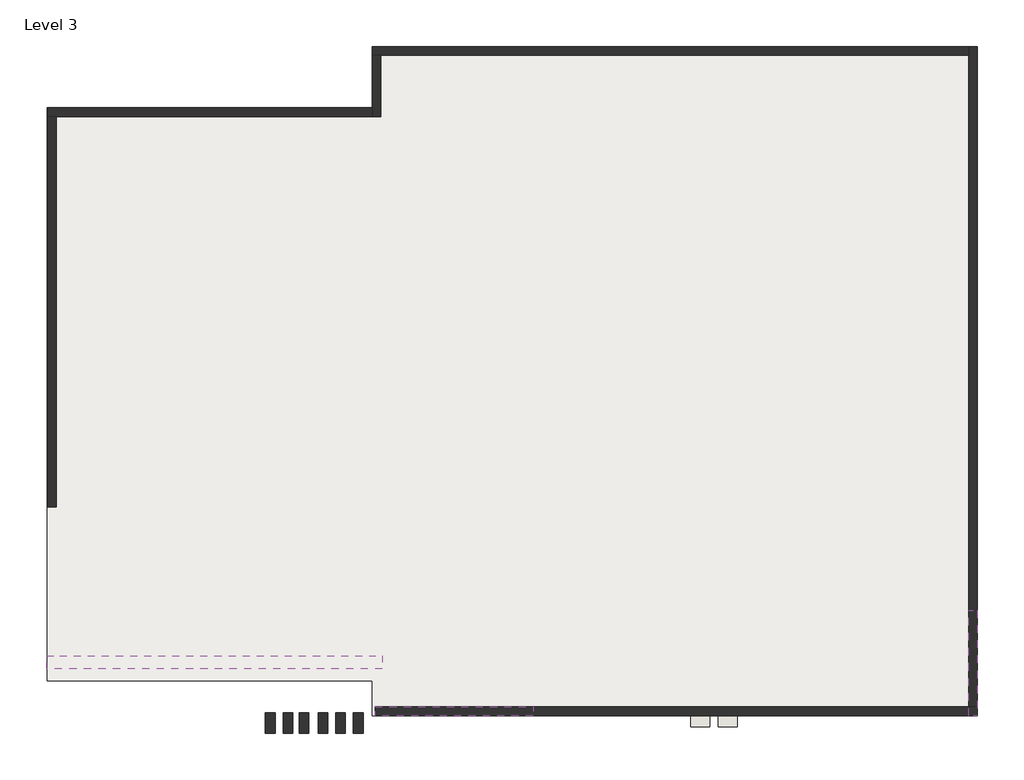
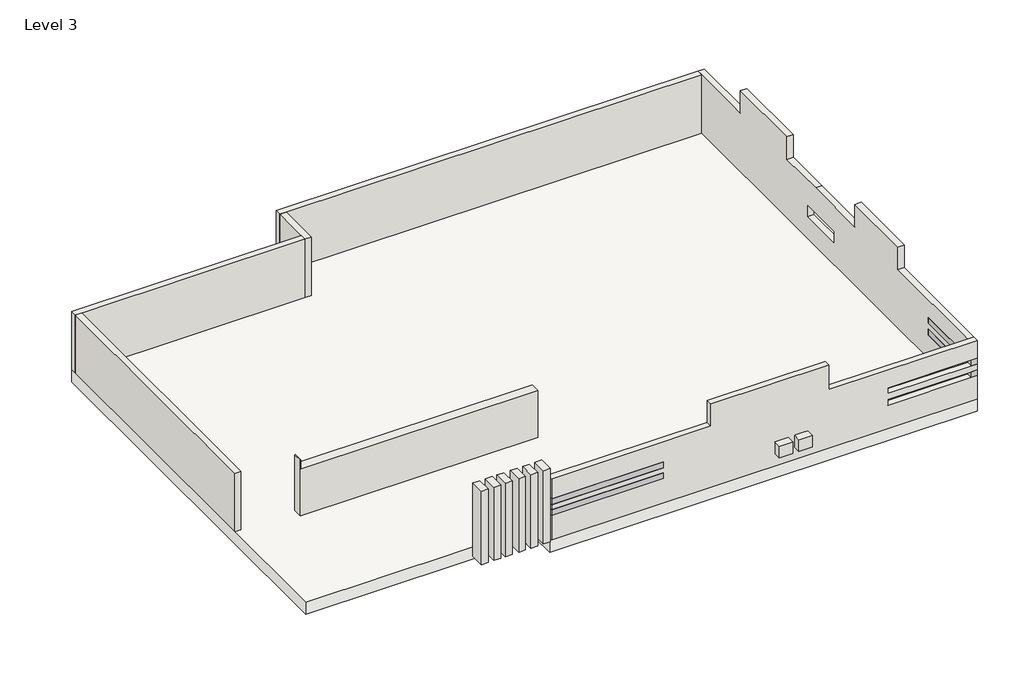
# One storey: 9 walls, 4 proxies, 1 roof.
"""IFC4 building model written with IfcOpenShell, lengths in millimetres."""

from ifc_helpers import new_model, si_unit, frame, origin, place, context, project, spatial, polyline, outline, extrude, faceted_brep, transform, mapped, element, save
from components import walls_3_walls_3_68a7d47a, walls_9_walls_9_54edce94

model = new_model("IFC4")

# Units and contexts
model_context = context("Model", 3, world=origin())
ifc_project = project(units=[si_unit("LENGTHUNIT", "METRE", prefix="MILLI")], contexts=[model_context])

# Site, building, storey
site = spatial("IfcSite", under=ifc_project)
building = spatial("IfcBuilding", under=site)
storey = spatial("IfcBuildingStorey", under=building, Name="Level 3", Elevation=7315.2)

# Proxies
placement = place(None, origin())
element("IfcBuildingElementProxy", 1, Name="Reveal", ObjectType="Reveal", at=placement, inside=storey, context=model_context, shape_type="SweptSolid", body=[
    extrude(outline(polyline([(2348.6271302, -3701.0259649), (2196.2271302, -3701.0259649), (2196.2271302, -1872.2259649), (2348.6271302, -1872.2259649), (2348.6271302, -3701.0259649)])), frame((0.0, 0.0, 8534.4), z_axis=(0.0, 0.0, 1.0), x_axis=(1.0, 0.0, 0.0)), (0.0, 0.0, 1.0), 152.4),
])
element("IfcBuildingElementProxy", 2, Name="Reveal", ObjectType="Reveal", at=placement, inside=storey, context=model_context, shape_type="SweptSolid", body=[
    extrude(outline(polyline([(-8116.1728698, -3701.0259649), (-8116.1728698, -3548.6259649), (-5372.9728698, -3548.6259649), (-5372.9728698, -3701.0259649), (-8116.1728698, -3701.0259649)])), frame((0.0, 0.0, 8536.4737715), z_axis=(0.0, 0.0, 1.0), x_axis=(1.0, 0.0, 0.0)), (0.0, 0.0, 1.0), 152.4),
])
element("IfcBuildingElementProxy", 3, Name="Reveal", ObjectType="Reveal", at=placement, inside=storey, context=model_context, shape_type="SweptSolid", body=[
    extrude(outline(polyline([(-8116.1728698, -3701.0259649), (-8116.1728698, -3548.6259649), (-5372.9728698, -3548.6259649), (-5372.9728698, -3701.0259649), (-8116.1728698, -3701.0259649)])), frame((0.0, 0.0, 8255.0001399), z_axis=(0.0, 0.0, 1.0), x_axis=(1.0, 0.0, 0.0)), (0.0, 0.0, 1.0), 152.4),
])
element("IfcBuildingElementProxy", 4, Name="Reveal", ObjectType="Reveal", at=placement, inside=storey, context=model_context, shape_type="SweptSolid", body=[
    extrude(outline(polyline([(2348.6271302, -3701.0259649), (2196.2271302, -3701.0259649), (2196.2271302, -1872.2259649), (2348.6271302, -1872.2259649), (2348.6271302, -3701.0259649)])), frame((0.0, 0.0, 8229.6), z_axis=(0.0, 0.0, 1.0), x_axis=(1.0, 0.0, 0.0)), (0.0, 0.0, 1.0), 152.4),
])

# Roof
element("IfcRoof", 5, ObjectType="Generic - 12\"", at=placement, inside=storey, context=model_context, shape_type="SweptSolid", body=[
    extrude(outline(polyline([(-13813.3305193, 6865.3740351), (-8166.9728698, 6865.3740351), (-8166.9728698, 7932.1740351), (2348.6271302, 7932.1740351), (2348.6271302, -3701.0259649), (-8166.9728698, -3701.0259649), (-8166.9728698, -3091.4259649), (-13813.3305193, -3091.4259649), (-13813.3305193, 6865.3740351)])), frame((0.0, 0.0, 7315.2), z_axis=(0.0, 0.0, 1.0), x_axis=(1.0, 0.0, 0.0)), (0.0, 0.0, 1.0), 304.8),
])

# Walls
element("IfcWall", 6, ObjectType="Generic - 6\"", at=placement, inside=storey, context=model_context, shape_type="Brep", body=[
    faceted_brep([(2348.6271302, -3701.0259649, 9144.0), (-1308.9728698, -3701.0259649, 9144.0), (-1308.9728698, -3701.0259649, 9785.7694166), (-4204.5728698, -3701.0259649, 9785.7694166), (-4204.5728698, -3701.0259649, 9212.8470483), (-8116.1728698, -3701.0259649, 9212.8470483), (-8116.1728698, -3701.0259649, 8688.8737715), (-5372.9728698, -3701.0259649, 8688.8737715), (-5372.9728698, -3701.0259649, 8536.4737715), (-8116.1728698, -3701.0259649, 8536.4737715), (-8116.1728698, -3701.0259649, 8407.4001399), (-5372.9728698, -3701.0259649, 8407.4001399), (-5372.9728698, -3701.0259649, 8255.0001399), (-8116.1728698, -3701.0259649, 8255.0001399), (-8116.1728698, -3701.0259649, 7617.5521516), (2348.6271302, -3701.0259649, 7617.5521516), (2348.6271302, -3701.0259649, 8229.6), (2196.2271302, -3701.0259649, 8229.6), (138.8271302, -3701.0259649, 8229.6), (138.8271302, -3701.0259649, 8380.7760758), (2196.2271302, -3701.0259649, 8380.7760758), (2196.2271302, -3701.0259649, 8382.0), (2348.6271302, -3701.0259649, 8382.0), (2348.6271302, -3701.0259649, 8534.4), (2196.2271302, -3701.0259649, 8534.4), (138.8271302, -3701.0259649, 8534.4), (138.8271302, -3701.0259649, 8686.8), (2196.2271302, -3701.0259649, 8686.8), (2348.6271302, -3701.0259649, 8686.8), (-1308.9728698, -3548.6259649, 9144.0), (2196.2271302, -3548.6259649, 9144.0), (2348.6271302, -3548.6259649, 9144.0), (2348.6271302, -3548.6259649, 8686.8), (2196.2271302, -3548.6259649, 8686.8), (138.8271302, -3548.6259649, 8686.8), (138.8271302, -3548.6259649, 8534.4), (2196.2271302, -3548.6259649, 8534.4), (2348.6271302, -3548.6259649, 8534.4), (2348.6271302, -3548.6259649, 8382.0), (2196.2271302, -3548.6259649, 8382.0), (2196.2271302, -3548.6259649, 8380.7760758), (138.8271302, -3548.6259649, 8380.7760758), (138.8271302, -3548.6259649, 8229.6), (2196.2271302, -3548.6259649, 8229.6), (2348.6271302, -3548.6259649, 8229.6), (2348.6271302, -3548.6259649, 7620.0), (2348.6271302, -3548.6259649, 7617.5521516), (-8116.1728698, -3548.6259649, 7617.5521516), (-8116.1728698, -3548.6259649, 8255.0001399), (-5372.9728698, -3548.6259649, 8255.0001399), (-5372.9728698, -3548.6259649, 8407.4001399), (-8116.1728698, -3548.6259649, 8407.4001399), (-8116.1728698, -3548.6259649, 8536.4737715), (-5372.9728698, -3548.6259649, 8536.4737715), (-5372.9728698, -3548.6259649, 8688.8737715), (-8116.1728698, -3548.6259649, 8688.8737715), (-8116.1728698, -3548.6259649, 9212.8470483), (-4204.5728698, -3548.6259649, 9212.8470483), (-4204.5728698, -3548.6259649, 9785.7694166), (-1308.9728698, -3548.6259649, 9785.7694166)], [[[0, 1, 2, 3, 4, 5, 6, 7, 8, 9, 10, 11, 12, 13, 14, 15, 16, 17, 18, 19, 20, 21, 22, 23, 24, 25, 26, 27, 28]], [[29, 30, 31, 32, 33, 34, 35, 36, 37, 38, 39, 40, 41, 42, 43, 44, 45, 46, 47, 48, 49, 50, 51, 52, 53, 54, 55, 56, 57, 58, 59]], [[1, 0, 31, 30, 29]], [[2, 1, 29, 59]], [[3, 2, 59, 58]], [[4, 3, 58, 57]], [[5, 4, 57, 56]], [[15, 14, 47, 46]], [[53, 8, 7, 54]], [[54, 7, 6, 55]], [[8, 53, 52, 9]], [[49, 12, 11, 50]], [[50, 11, 10, 51]], [[12, 49, 48, 13]], [[5, 56, 55, 6]], [[47, 14, 13, 48]], [[51, 10, 9, 52]], [[21, 39, 38, 22]], [[39, 21, 20, 40]], [[42, 18, 17, 16, 44, 43]], [[19, 18, 42, 41]], [[19, 41, 40, 20]], [[35, 25, 24, 23, 37, 36]], [[26, 25, 35, 34]], [[26, 34, 33, 32, 28, 27]], [[16, 15, 46, 45, 44]], [[37, 23, 22, 38]], [[0, 28, 32, 31]]]),
])
element("IfcWall", 7, ObjectType="Generic - 6\"", at=placement, inside=storey, context=model_context, shape_type="Brep", body=[
    faceted_brep([(2348.6271302, -3548.6259649, 7620.0), (2348.6271302, 7932.1740351, 7620.0), (2348.6271302, 7932.1740351, 9144.0), (2348.6271302, 6128.7740351, 9144.0), (2348.6271302, 6128.7740351, 9731.3133194), (2348.6271302, 4147.5740351, 9731.3133194), (2348.6271302, 4147.5740351, 9144.0), (2348.6271302, 2928.3740351, 9144.0), (2348.6271302, 1251.9740351, 9144.0), (2348.6271302, 1251.9740351, 9731.3133194), (2348.6271302, -576.8259649, 9731.3133194), (2348.6271302, -576.8259649, 9144.0), (2348.6271302, -3548.6259649, 9144.0), (2348.6271302, -3548.6259649, 8686.8), (2348.6271302, -1872.2259649, 8686.8), (2348.6271302, -1872.2259649, 8534.4), (2348.6271302, -3548.6259649, 8534.4), (2348.6271302, -3548.6259649, 8382.0), (2348.6271302, -1872.2259649, 8382.0), (2348.6271302, -1872.2259649, 8229.6), (2348.6271302, -3548.6259649, 8229.6), (2348.6271302, 3260.506606, 8479.0034325), (2348.6271302, 3260.506606, 8199.6034325), (2348.6271302, 2142.906606, 8199.6034325), (2348.6271302, 2142.906606, 8479.0034325), (2196.2271302, 7932.1740351, 7620.0), (2196.2271302, 7779.7740351, 7620.0), (2196.2271302, -3548.6259649, 7620.0), (2196.2271302, -3548.6259649, 8229.6), (2196.2271302, -1872.2259649, 8229.6), (2196.2271302, -1872.2259649, 8382.0), (2196.2271302, -3548.6259649, 8382.0), (2196.2271302, -3548.6259649, 8534.4), (2196.2271302, -1872.2259649, 8534.4), (2196.2271302, -1872.2259649, 8686.8), (2196.2271302, -3548.6259649, 8686.8), (2196.2271302, -3548.6259649, 9144.0), (2196.2271302, -576.8259649, 9144.0), (2196.2271302, -576.8259649, 9731.3133194), (2196.2271302, 1251.9740351, 9731.3133194), (2196.2271302, 1251.9740351, 9144.0), (2196.2271302, 2928.3740351, 9144.0), (2196.2271302, 4147.5740351, 9144.0), (2196.2271302, 4147.5740351, 9731.3133194), (2196.2271302, 6128.7740351, 9731.3133194), (2196.2271302, 6128.7740351, 9144.0), (2196.2271302, 7779.7740351, 9144.0), (2196.2271302, 7932.1740351, 9144.0), (2196.2271302, 3260.506606, 8199.6034325), (2196.2271302, 3260.506606, 8479.0034325), (2196.2271302, 2142.906606, 8479.0034325), (2196.2271302, 2142.906606, 8199.6034325)], [[[0, 1, 2, 3, 4, 5, 6, 7, 8, 9, 10, 11, 12, 13, 14, 15, 16, 17, 18, 19, 20], [21, 22, 23, 24]], [[25, 26, 27, 28, 29, 30, 31, 32, 33, 34, 35, 36, 37, 38, 39, 40, 41, 42, 43, 44, 45, 46, 47], [48, 49, 50, 51]], [[2, 1, 25, 47]], [[1, 0, 27, 26, 25]], [[12, 11, 37, 36]], [[33, 15, 14, 34]], [[34, 14, 13, 35]], [[15, 33, 32, 16]], [[3, 2, 47, 46, 45]], [[4, 3, 45, 44]], [[5, 4, 44, 43]], [[6, 5, 43, 42]], [[7, 6, 42, 41]], [[8, 7, 41, 40]], [[9, 8, 40, 39]], [[10, 9, 39, 38]], [[11, 10, 38, 37]], [[29, 19, 18, 30]], [[30, 18, 17, 31]], [[19, 29, 28, 20]], [[27, 0, 20, 28]], [[12, 36, 35, 13]], [[16, 32, 31, 17]], [[22, 21, 49, 48]], [[23, 22, 48, 51]], [[24, 23, 51, 50]], [[21, 24, 50, 49]]]),
])
element("IfcWall", 8, ObjectType="Generic - 6\"", at=placement, inside=storey, context=model_context, shape_type="Brep", body=[
    faceted_brep([(2196.2271302, 7932.1740351, 7620.0), (-8166.9728698, 7932.1740351, 7620.0), (-8166.9728698, 7932.1740351, 9144.0), (2196.2271302, 7932.1740351, 9144.0), (2196.2271302, 7779.7740351, 7620.0), (2196.2271302, 7779.7740351, 9144.0), (-8014.5728698, 7779.7740351, 9144.0), (-8166.9728698, 7779.7740351, 9144.0), (-8166.9728698, 7779.7740351, 7620.0), (-8014.5728698, 7779.7740351, 7620.0)], [[[0, 1, 2, 3]], [[4, 5, 6, 7, 8, 9]], [[0, 3, 5, 4]], [[2, 1, 8, 7]], [[1, 0, 4, 9, 8]], [[3, 2, 7, 6, 5]]]),
])
element("IfcWall", 9, ObjectType="Generic - 6\"", at=placement, inside=storey, context=model_context, shape_type="Brep", body=[
    faceted_brep([(-8166.9728698, 7779.7740351, 7620.0), (-8166.9728698, 6865.3740351, 7620.0), (-8166.9728698, 6712.9740351, 7620.0), (-8166.9728698, 6712.9740351, 9144.0), (-8166.9728698, 6865.3740351, 9144.0), (-8166.9728698, 7779.7740351, 9144.0), (-8014.5728698, 7779.7740351, 7620.0), (-8014.5728698, 7779.7740351, 9144.0), (-8014.5728698, 6712.9740351, 9144.0), (-8014.5728698, 6712.9740351, 7620.0)], [[[0, 1, 2, 3, 4, 5]], [[6, 7, 8, 9]], [[2, 1, 0, 6, 9]], [[5, 4, 3, 8, 7]], [[0, 5, 7, 6]], [[3, 2, 9, 8]]]),
])
element("IfcWall", 10, ObjectType="Generic - 6\"", at=placement, inside=storey, context=model_context, shape_type="Brep", body=[
    faceted_brep([(-8166.9728698, 6865.3740351, 7620.0), (-13806.9805193, 6865.3740351, 7620.0), (-13806.9805193, 6865.3740351, 9144.0), (-8166.9728698, 6865.3740351, 9144.0), (-8166.9728698, 6712.9740351, 7620.0), (-8166.9728698, 6712.9740351, 9144.0), (-13654.5805193, 6712.9740351, 9144.0), (-13806.9805193, 6712.9740351, 9144.0), (-13806.9805193, 6712.9740351, 7620.0), (-13654.5805193, 6712.9740351, 7620.0)], [[[0, 1, 2, 3]], [[4, 5, 6, 7, 8, 9]], [[1, 0, 4, 9, 8]], [[3, 2, 7, 6, 5]], [[0, 3, 5, 4]], [[2, 1, 8, 7]]]),
])
element("IfcWall", 11, ObjectType="Generic - 6\"", at=placement, inside=storey, context=model_context, shape_type="SweptSolid", body=[
    extrude(outline(polyline([(-13806.9805193, -68.8259649), (-13806.9805193, 6712.9740351), (-13654.5805193, 6712.9740351), (-13654.5805193, -68.8259649), (-13806.9805193, -68.8259649)])), frame((0.0, 0.0, 7620.0), z_axis=(0.0, 0.0, 1.0), x_axis=(1.0, 0.0, 0.0)), (0.0, 0.0, 1.0), 1524.0),
])
element("IfcWall", 12, ObjectType="Generic - 8\" - Filled", at=placement, inside=storey, context=model_context, shape_type="Brep", body=[
    faceted_brep([(-13824.8228698, -2888.2259649, 9753.6), (-7989.1728698, -2888.2259649, 9753.6), (-7989.1728698, -2888.2259649, 10972.8), (-13810.1555193, -2888.2259649, 10972.8), (-13810.1555193, -2888.2259649, 11202.4428486), (-13824.8228698, -2888.2259649, 11202.4428486), (-13824.8228698, -2659.6259649, 9753.6), (-13824.8228698, -2659.6259649, 11194.4859918), (-13824.8228698, -2659.6259649, 11202.4428486), (-13810.1555193, -2659.6259649, 11202.4428486), (-13810.1555193, -2659.6259649, 11194.4859918), (-13810.1555193, -2659.6259649, 10972.8), (-13596.2228698, -2659.6259649, 10972.8), (-8217.7728698, -2659.6259649, 10972.8), (-7989.1728698, -2659.6259649, 10972.8), (-7989.1728698, -2659.6259649, 9753.6), (-13596.2228698, -2659.6259649, 9753.6)], [[[0, 1, 2, 3, 4, 5]], [[6, 7, 8, 9, 10, 11, 12, 13, 14, 15, 16]], [[1, 0, 6, 16, 15]], [[0, 5, 8, 7, 6]], [[2, 1, 15, 14]], [[5, 4, 9, 8]], [[9, 4, 3, 11, 10]], [[3, 2, 14, 13, 12, 11]]]),
])
walls_3_walls_3_shape = walls_3_walls_3_68a7d47a(model_context)
element("IfcWall", 13, ObjectType="Walls 3 : Walls 3", at=placement, inside=storey, context=model_context, shape_type="MappedRepresentation", body=[
    mapped(walls_3_walls_3_shape, transform((0.0, 0.0, 0.0), x_axis=(1.0, 0.0, 0.0), y_axis=(0.0, 1.0, 0.0), z_axis=(0.0, 0.0, 1.0))),
])
walls_9_walls_9_shape = walls_9_walls_9_54edce94(model_context)
element("IfcWall", 14, ObjectType="Walls 9 : Walls 9", at=placement, inside=storey, context=model_context, shape_type="MappedRepresentation", body=[
    mapped(walls_9_walls_9_shape, transform((0.0, 0.0, 0.0), x_axis=(1.0, 0.0, 0.0), y_axis=(0.0, 1.0, 0.0), z_axis=(0.0, 0.0, 1.0))),
])

save(model, "model.ifc")

# Revit data of these elements
# Type "Generic - 12\""
#   Assembly Code = "B1020"
#   Layers, outside or top first: 1' - 0" no material (function 1)
# Type "Generic - 6\""
#   Assembly Code = "B2010"
#   Layers, outside or top first: 0' - 6" no material (function 1)
# Type "Generic - 8\" - Filled"
#   Assembly Code = "B2010"
#   Layers, outside or top first: 0' - 9" no material (function 1)
# Element 5 (IfcRoof, "Generic - 12\"")
#   built-in parameter 1001705 = 25 (stored number, unit not read)
#   built-in parameter 1001710 = 33615
#   Phase Created = New Construction
#   Materials on its faces: "Default Roof"
# Element 6 (IfcWall, "Generic - 6\"")
#   built-in parameter 1001111 = 1' - 0"
#   Top Offset = 0' - 0"
#   Base Offset = 1' - 0"
#   Unconnected Height = 5' - 2.71051"
#   wall height = 5' - 2.71051"
#   Phase Created = New Construction
#   Base Constraint = Level 3
#   Materials on its faces: "Default Wall"
# Elements 7, 8, 9, 10, 11 (IfcWall, "Generic - 6\"")
#   built-in parameter 1001111 = 1' - 0"
#   Top Offset = 0' - 0"
#   Base Offset = 1' - 0"
#   Unconnected Height = 5' - 0"
#   wall height = 5' - 0"
#   Phase Created = New Construction
#   Base Constraint = Level 3
#   Materials on its faces: "Default Wall"
# Element 12 (IfcWall, "Generic - 8\" - Filled")
#   built-in parameter 1001111 = 8' - 0"
#   Top Offset = 0' - 0"
#   Base Offset = 8' - 0"
#   Unconnected Height = 4' - 9.04106"
#   wall height = 4' - 9.04106"
#   Phase Created = New Construction
#   Base Constraint = Level 3
#   Materials on its faces: "Default Wall"
# Element 13 (IfcWall, "Walls 3 : Walls 3")
#   Phase Created = New Construction
#   Materials on its faces: "Default Wall"
# Element 14 (IfcWall, "Walls 9 : Walls 9")
#   Phase Created = New Construction
#   Materials on its faces: "Default Wall"
# Materials
#   "Default Roof": colour RGB 88 101 114, transparency 0
#   "Default Wall": colour RGB 128 128 128, transparency 0
